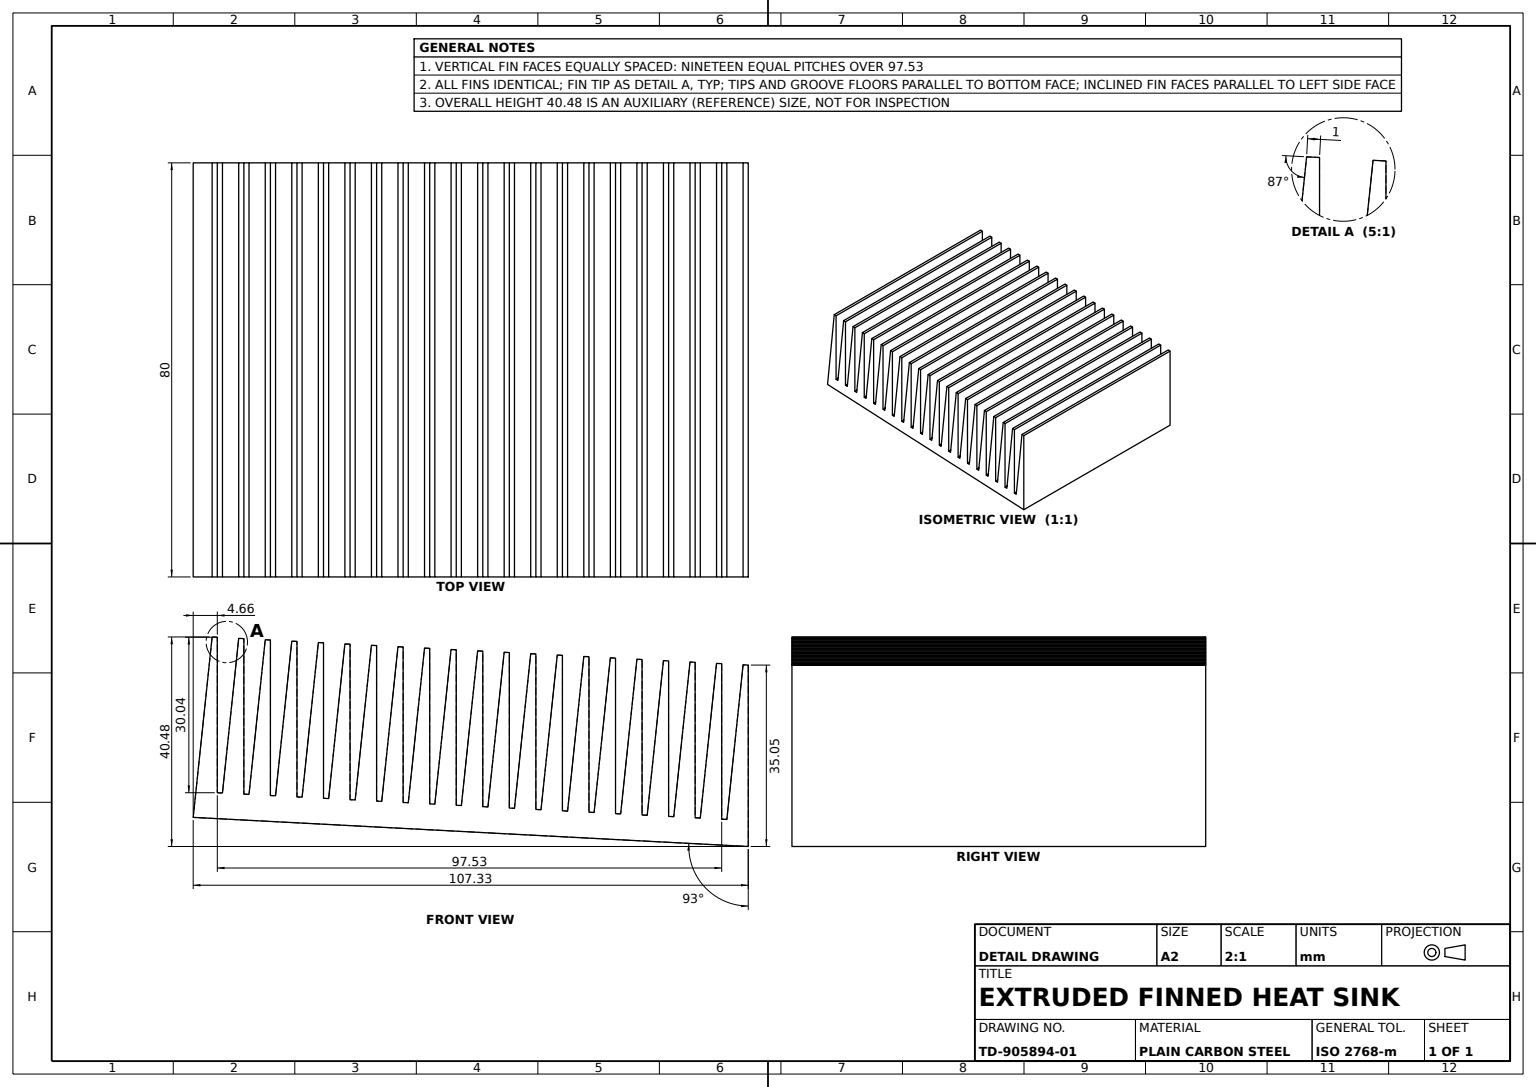
SolidWorks part; units mm, degrees
material "Plain Carbon Steel"
ref_plane "Front Plane" through (0, 0, 0) normal (0, 0, 1) x (1, 0, 0)
ref_plane "Top Plane" through (0, 0, 0) normal (0, 1, 0) x (1, 0, 0)
ref_plane "Right Plane" through (0, 0, 0) normal (1, 0, 0) x (0, 0, -1)
sketch "Heat Sink Profile 20 Fins" plane through (0, 0, 0) normal (0, 1, 0) x (1, 0, 0)
  line L0 (-39.9975, 17.548) -> (-38.9975, 17.548)
  line L2 (-39.9975, 17.548) -> (-41.8318, -17.452)
  line L5 (-38.9975, 17.548) -> (-37.4253, -12.452)
  line L6 (-37.4253, -12.452) -> (-36.4253, -12.452)
  line L7 (-36.4253, -12.452) -> (-34.853, 17.548)
  line L8 (-34.853, 17.548) -> (-33.853, 17.548)
  line L9 (-33.853, 17.548) -> (-32.2808, -12.452)
  line L10 (-56.3137, 17.548) -> (-13.3923, 17.548) construction
  line L11 (-31.2853, -12.452) -> (-29.713, 17.548)
  line L12 (-28.713, 17.548) -> (-27.1408, -12.452)
  line L13 (-32.2853, -12.452) -> (-31.2853, -12.452)
  line L14 (-29.713, 17.548) -> (-28.713, 17.548)
  line L15 (-26.1453, -12.452) -> (-24.573, 17.548)
  line L16 (-23.573, 17.548) -> (-22.0008, -12.452)
  line L17 (-27.1453, -12.452) -> (-26.1453, -12.452)
  line L18 (-24.573, 17.548) -> (-23.573, 17.548)
  line L19 (-21.0053, -12.452) -> (-19.433, 17.548)
  line L20 (-18.433, 17.548) -> (-16.8608, -12.452)
  line L21 (-22.0053, -12.452) -> (-21.0053, -12.452)
  line L22 (-19.433, 17.548) -> (-18.433, 17.548)
  line L23 (-15.8653, -12.452) -> (-14.293, 17.548)
  line L24 (-13.293, 17.548) -> (-11.7208, -12.452)
  line L25 (-16.8653, -12.452) -> (-15.8653, -12.452)
  line L26 (-14.293, 17.548) -> (-13.293, 17.548)
  line L27 (-10.7253, -12.452) -> (-9.153, 17.548)
  line L28 (-8.153, 17.548) -> (-6.5808, -12.452)
  line L29 (-11.7253, -12.452) -> (-10.7253, -12.452)
  line L30 (-9.153, 17.548) -> (-8.153, 17.548)
  line L31 (-5.5853, -12.452) -> (-4.013, 17.548)
  line L32 (-3.013, 17.548) -> (-1.4408, -12.452)
  line L33 (-6.5853, -12.452) -> (-5.5853, -12.452)
  line L34 (-4.013, 17.548) -> (-3.013, 17.548)
  line L35 (-0.4453, -12.452) -> (1.127, 17.548)
  line L36 (2.127, 17.548) -> (3.6992, -12.452)
  line L37 (-1.4453, -12.452) -> (-0.4453, -12.452)
  line L38 (1.127, 17.548) -> (2.127, 17.548)
  line L39 (4.6947, -12.452) -> (6.267, 17.548)
  line L40 (7.267, 17.548) -> (8.8392, -12.452)
  line L41 (3.6947, -12.452) -> (4.6947, -12.452)
  line L42 (6.267, 17.548) -> (7.267, 17.548)
  line L43 (9.8347, -12.452) -> (11.407, 17.548)
  line L44 (12.407, 17.548) -> (13.9792, -12.452)
  line L45 (8.8347, -12.452) -> (9.8347, -12.452)
  line L46 (11.407, 17.548) -> (12.407, 17.548)
  line L47 (14.9747, -12.452) -> (16.547, 17.548)
  line L48 (17.547, 17.548) -> (19.1192, -12.452)
  line L49 (13.9747, -12.452) -> (14.9747, -12.452)
  line L50 (16.547, 17.548) -> (17.547, 17.548)
  line L51 (20.1147, -12.452) -> (21.687, 17.548)
  line L52 (22.687, 17.548) -> (24.2592, -12.452)
  line L53 (19.1147, -12.452) -> (20.1147, -12.452)
  line L54 (21.687, 17.548) -> (22.687, 17.548)
  line L55 (25.2547, -12.452) -> (26.827, 17.548)
  line L56 (27.827, 17.548) -> (29.3992, -12.452)
  line L57 (24.2547, -12.452) -> (25.2547, -12.452)
  line L58 (26.827, 17.548) -> (27.827, 17.548)
  line L59 (30.3947, -12.452) -> (31.967, 17.548)
  line L60 (32.967, 17.548) -> (34.5392, -12.452)
  line L61 (29.3947, -12.452) -> (30.3947, -12.452)
  line L62 (31.967, 17.548) -> (32.967, 17.548)
  line L63 (35.5347, -12.452) -> (37.107, 17.548)
  line L64 (38.107, 17.548) -> (39.6792, -12.452)
  line L65 (34.5347, -12.452) -> (35.5347, -12.452)
  line L66 (37.107, 17.548) -> (38.107, 17.548)
  line L67 (40.6747, -12.452) -> (42.247, 17.548)
  line L68 (43.247, 17.548) -> (44.8192, -12.452)
  line L69 (39.6747, -12.452) -> (40.6747, -12.452)
  line L70 (42.247, 17.548) -> (43.247, 17.548)
  line L71 (45.8147, -12.452) -> (47.387, 17.548)
  line L72 (48.387, 17.548) -> (49.9592, -12.452)
  line L73 (44.8147, -12.452) -> (45.8147, -12.452)
  line L74 (47.387, 17.548) -> (48.387, 17.548)
  line L75 (50.9547, -12.452) -> (52.527, 17.548)
  line L76 (53.527, 17.548) -> (55.0992, -12.452)
  line L77 (49.9547, -12.452) -> (50.9547, -12.452)
  line L78 (52.527, 17.548) -> (53.527, 17.548)
  line L79 (56.0947, -12.452) -> (57.667, 17.548)
  line L80 (58.667, 17.548) -> (60.2392, -12.452)
  line L81 (55.0947, -12.452) -> (56.0947, -12.452)
  line L82 (57.667, 17.548) -> (58.667, 17.548)
  line L83 (61.2347, -12.452) -> (62.807, 17.548)
  line L84 (63.807, 17.548) -> (65.6413, -17.452)
  line L85 (60.2347, -12.452) -> (61.2347, -12.452)
  line L86 (62.807, 17.548) -> (63.807, 17.548)
  line L87 (-41.8318, -17.452) -> (65.6413, -17.452)
  point P0 (0, 0)
  dimension "D2" = 93
  dimension "D3" = 5
  dimension "D4" = 1
  dimension "D5" = 1
  dimension "D6" = 1
  dimension "D7" = 87
  dimension "D8" = 93
  dimension "D9" = 87
  dimension "D10" = 0
  dimension "D11" = 35
  dimension "D12" = 87
  dimension "D13" = 87
  dimension "D14" = 93
  dimension "D15" = 30.0412
  dimension "D16" = 9.551
  dimension "D17" = 20
  dimension "D18" = 9.5465
  dimension "D19" = 41.8318
  dimension "D20" = 17.452
extrude "Heat Sink Body Extrude 80mm" add sketch "Heat Sink Profile 20 Fins" along normal blind 80
